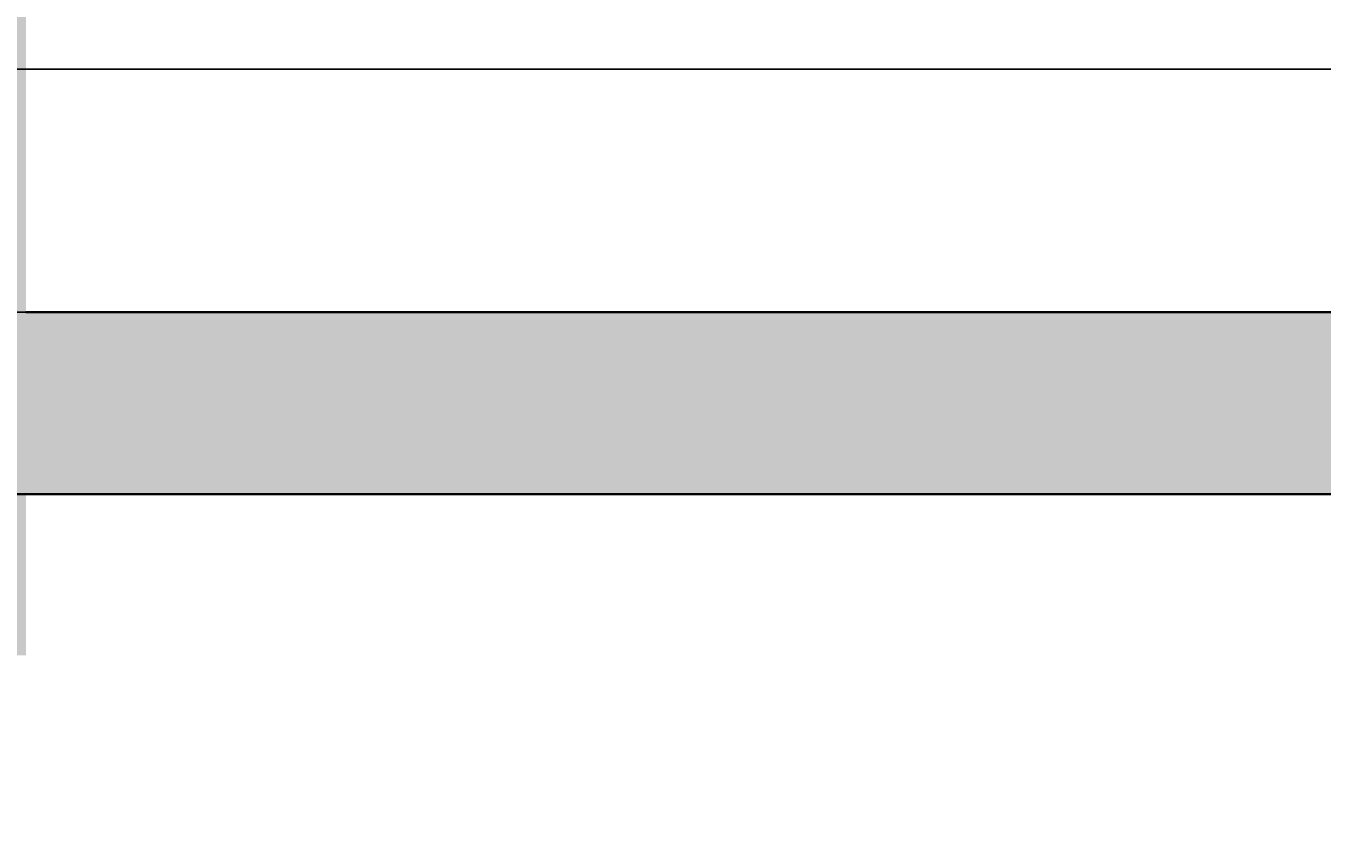
# Model space of a CAD drawing. Units: inches. Extents: x 1998 to 2588, y 1139 to 1977.
# Tile 10 of 134: x 2115 to 2147, y 1576 to 1596. Entities that reach past the tile are written whole.
import ezdxf

# ---------------------------------------------------------------- set-up
doc = ezdxf.new("R2010")
doc.units = ezdxf.units.IN
for name, color, linetype, lineweight in [('A-ANNO-DIMS', 2, 'Continuous', 18), ('A-WALL-PATT', 252, 'Continuous', 13), ('WALL', 200, 'Continuous', 35)]:
    doc.layers.add(name, color=color, linetype=linetype, lineweight=lineweight)
doc.styles.get("Standard").update_dxf_attribs({"font": 'arial.ttf'})
doc.dimstyles.get("Standard").update_dxf_attribs({"dimtxt": 0.18, "dimasz": 0.18, "dimexe": 0.18, "dimexo": 0.0625, "dimgap": 0.09, "dimtad": 0, "dimtih": 1, "dimtoh": 1, "dimdec": 4, "dimzin": 0, "dimdsep": 46, "dimtxsty": 'Standard', "dimcen": 0.09, "dimadec": 0, "dimazin": 0, "dimtfac": 1, "dimtdec": 4, "dimtofl": 0, "dimtmove": 0, "dimatfit": 3, "dimfxl": 1, "dimtolj": 1, "dimtzin": 0, "dimarcsym": 0})

# ---------------------------------------------------------------- blocks, each defined once
blk = doc.blocks.new('*D30')
at = {"layer": 'A-ANNO-DIMS', "color": 0, "lineweight": -2, "transparency": 16777216}
for p, q in [((2407.91, 1636.732), (1997.843, 1636.732)), ((1998.023, 1636.552), (1998.023, 1615.913)), ((1998.023, 1594.912), (1998.023, 1615.552)), ((2407.91, 1594.732), (1997.843, 1594.732))]:
    blk.add_line(p, q, dxfattribs=at)
at = {"layer": 'A-ANNO-DIMS', "color": 0, "transparency": 16777216}
for points in [[(1997.993, 1636.552), (1998.053, 1636.552), (1998.023, 1636.732)], [(1997.993, 1594.912), (1998.053, 1594.912), (1998.023, 1594.732)]]:
    blk.add_solid(points, dxfattribs=at)
at = {"layer": 'Defpoints', "color": 0, "transparency": 16777216}
for p in [(1998.023, 1636.732), (2407.973, 1636.732), (2407.973, 1594.732)]:
    blk.add_point(p, dxfattribs=at)
at = {"layer": 'A-ANNO-DIMS', "color": 0, "transparency": 16777216, "insert": (1998.023, 1615.732), "char_height": 0.18, "attachment_point": 5}
blk.add_mtext('\\A1;42', dxfattribs=at)
blk = doc.blocks.new('*D34')
at = {"layer": 'A-ANNO-DIMS', "color": 0, "lineweight": -2, "transparency": 16777216}
for p, q in [((2407.91, 1594.732), (1997.843, 1594.732)), ((1998.023, 1594.552), (1998.023, 1558.913)), ((1998.023, 1522.912), (1998.023, 1558.552)), ((2407.91, 1522.732), (1997.843, 1522.732))]:
    blk.add_line(p, q, dxfattribs=at)
at = {"layer": 'A-ANNO-DIMS', "color": 0, "transparency": 16777216}
for points in [[(1997.993, 1594.552), (1998.053, 1594.552), (1998.023, 1594.732)], [(1997.993, 1522.912), (1998.053, 1522.912), (1998.023, 1522.732)]]:
    blk.add_solid(points, dxfattribs=at)
at = {"layer": 'Defpoints', "color": 0, "transparency": 16777216}
for p in [(1998.023, 1594.732), (2407.973, 1594.732), (2407.973, 1522.732)]:
    blk.add_point(p, dxfattribs=at)
at = {"layer": 'A-ANNO-DIMS', "color": 0, "transparency": 16777216, "insert": (1998.023, 1558.732), "char_height": 0.18, "attachment_point": 5}
blk.add_mtext('\\A1;72', dxfattribs=at)
blk = doc.blocks.new('*D35')
at = {"layer": 'A-ANNO-DIMS', "color": 0, "lineweight": -2, "transparency": 16777216}
for p, q in [((2148.392, 1612.732), (1997.843, 1612.732)), ((1998.023, 1612.552), (1998.023, 1600.913)), ((1998.023, 1588.912), (1998.023, 1600.552)), ((2148.392, 1588.732), (1997.843, 1588.732))]:
    blk.add_line(p, q, dxfattribs=at)
at = {"layer": 'A-ANNO-DIMS', "color": 0, "transparency": 16777216}
for points in [[(1997.993, 1612.552), (1998.053, 1612.552), (1998.023, 1612.732)], [(1997.993, 1588.912), (1998.053, 1588.912), (1998.023, 1588.732)]]:
    blk.add_solid(points, dxfattribs=at)
at = {"layer": 'Defpoints', "color": 0, "transparency": 16777216}
for p in [(1998.023, 1612.732), (2148.455, 1612.732), (2148.455, 1588.732)]:
    blk.add_point(p, dxfattribs=at)
at = {"layer": 'A-ANNO-DIMS', "color": 0, "transparency": 16777216, "insert": (1998.023, 1600.732), "char_height": 0.18, "attachment_point": 5}
blk.add_mtext('\\A1;24', dxfattribs=at)

msp = doc.modelspace()

# ---------------------------------------------------------------- hatches: boundary and pattern name
at = {"layer": 'A-WALL-PATT'}
h = msp.add_hatch(color=256, dxfattribs=at)
h.dxf.hatch_style = 1
h.paths.add_polyline_path([(2222.9729, 1888.7324), (2099.4125, 1888.7324), (2099.4125, 1879.7324), (2222.9729, 1879.7324)])
h.paths.add_polyline_path([(2096.9729, 1868.3278), (2087.9729, 1868.3278), (2087.9729, 1775.637), (2096.9729, 1775.637)])
h.paths.add_polyline_path([(2227.4729, 1868.3278), (2222.9729, 1868.3278), (2222.9729, 1774.3318), (2227.4729, 1774.3318)])
h.paths.add_polyline_path([(2188.3019, 1759.7324), (2138.6074, 1759.7324), (2099.4125, 1759.7324), (2099.4125, 1755.2324), (2176.9729, 1755.2324), (2188.3019, 1755.2324)])
h.paths.add_polyline_path([(2087.9729, 1759.7324), (2059.4729, 1759.7324), (2059.4729, 1702.7324), (2087.9729, 1702.7324), (2087.9729, 1707.2324), (2063.9729, 1707.2324), (2063.9729, 1755.2324), (2087.9729, 1755.2324)])
h.paths.add_polyline_path([(2096.9729, 1755.2324), (2087.9729, 1755.2324), (2087.9729, 1707.2324), (2096.9729, 1707.2324)])
h.paths.add_polyline_path([(2187.0461, 1707.2324), (2105.9729, 1707.2324), (2096.9729, 1707.2324), (2087.9729, 1707.2324), (2087.9729, 1702.7324), (2105.9729, 1702.7324), (2114.9729, 1702.7324), (2187.0461, 1702.7324)])
h.paths.add_polyline_path([(2181.4729, 1719.2028), (2176.9729, 1719.2028), (2176.9729, 1707.2324), (2181.4729, 1707.2324)])
h.paths.add_polyline_path([(2216.0332, 1588.7324), (2114.9729, 1588.7324), (2105.9729, 1588.7324), (2105.9729, 1584.2324), (2216.0332, 1584.2324)])
h.paths.add_polyline_path([(2077.691, 1588.7324), (2061.4729, 1588.7324), (2061.4729, 1584.2324), (2077.691, 1584.2324)])
h.paths.add_polyline_path([(2105.9729, 1588.7324), (2098.0956, 1588.7324), (2098.0956, 1584.2324), (2105.9729, 1584.2324)])
h.paths.add_polyline_path([(2114.9729, 1596.2642), (2110.1012, 1596.2642), (2105.9729, 1596.2642), (2105.9729, 1588.7324), (2114.9729, 1588.7324)])
h.paths.add_polyline_path([(2114.9729, 1584.2324), (2105.9729, 1584.2324), (2105.9729, 1580.249), (2110.1012, 1580.249), (2114.9729, 1580.249)])
h.paths.add_polyline_path([(2114.9729, 1547.7716), (2110.1012, 1547.7716, -0.0318759), (2105.9729, 1548.035), (2105.9729, 1470.2324), (2108.3775, 1470.2324), (2108.3775, 1465.7324), (2186.2943, 1465.7324), (2186.2943, 1470.2324), (2114.9729, 1470.2324)])
h.paths.add_polyline_path([(2227.4729, 1584.2324), (2222.9729, 1584.2324), (2222.9729, 1486.137), (2227.4729, 1486.137)])
h.paths.add_polyline_path([(2295.4138, 1593.2324), (2227.4729, 1593.2324), (2227.4729, 1588.7324), (2295.4138, 1588.7324), (2295.4138, 1591.8729)])
h.paths.add_polyline_path([(2345.9729, 1627.1165), (2341.4729, 1627.1165), (2341.4729, 1593.2324), (2337.2869, 1593.2324), (2337.2869, 1591.8729), (2337.2869, 1588.7324), (2345.9729, 1588.7324)])
h.paths.add_polyline_path([(2291.9729, 1588.7324), (2287.4729, 1588.7324), (2287.4729, 1522.7324), (2291.9729, 1522.7324)])
h.paths.add_polyline_path([(2291.9729, 1522.7324), (2287.4729, 1522.7324), (2227.4729, 1522.7324), (2227.4729, 1518.2324), (2291.9729, 1518.2324)])
h.paths.add_polyline_path([(2295.7347, 1519.5919), (2295.7347, 1522.7324), (2291.9729, 1522.7324), (2291.9729, 1518.2324), (2295.7347, 1518.2324)])
h.paths.add_polyline_path([(2345.9729, 1522.7324), (2337.6078, 1522.7324), (2337.6078, 1519.5919), (2337.6078, 1518.2324), (2341.4729, 1518.2324), (2341.4729, 1488.5616), (2345.9729, 1488.5616)])
h.paths.add_polyline_path([(2345.9729, 1468.1569), (2341.4729, 1468.1569), (2341.4729, 1374.2324), (2227.4729, 1374.2324), (2227.4729, 1369.7324), (2345.9729, 1369.7324)])
h.paths.add_polyline_path([(2345.9729, 1369.7324), (2341.4729, 1369.7324), (2341.4729, 1362.2324), (2345.9729, 1362.2324)])
h.paths.add_polyline_path([(2345.9729, 1317.7324), (2345.9729, 1322.2324), (2341.4729, 1322.2324), (2341.4729, 1285.137), (2345.9729, 1285.137)], flags=17)
h.paths.add_polyline_path([(2356.2096, 1322.2324), (2345.9729, 1322.2324), (2345.9729, 1317.7324), (2356.2096, 1317.7324), (2356.2096, 1319.3088)], flags=17)
h.paths.add_polyline_path([(2393.9729, 1322.2324), (2375.6999, 1322.2324), (2375.6999, 1319.3088, -0.0202458), (2375.636, 1317.7324), (2393.9729, 1317.7324)], flags=17)
h.paths.add_polyline_path([(2398.4729, 1322.2324), (2393.9729, 1322.2324), (2393.9729, 1317.7324), (2393.9729, 1237.7324), (2345.9729, 1237.7324), (2345.9729, 1264.7324), (2341.4729, 1264.7324), (2341.4729, 1228.7324), (2393.9729, 1228.7324), (2482.7412, 1228.7324), (2482.7412, 1237.7324), (2398.4729, 1237.7324), (2398.4729, 1297.1029)])
h.paths.add_polyline_path([(2398.4729, 1362.2324), (2393.9729, 1362.2324), (2393.9729, 1357.7324), (2398.4729, 1357.7324)])
h.paths.add_polyline_path([(2345.9729, 1329.7549), (2341.4729, 1329.7549), (2341.4729, 1322.2324), (2345.9729, 1322.2324)])

# ---------------------------------------------------------------- linework, layer by layer
at = {"layer": 'WALL'}
for p, q in [((2216.0332, 1588.7324), (2114.9729, 1588.7324)), ((2227.4729, 1584.2324), (2105.9729, 1584.2324))]:
    msp.add_line(p, q, dxfattribs=at)

# ---------------------------------------------------------------- dimensions: what is measured, and where the dimension line sits
at = {"layer": 'A-ANNO-DIMS'}
for base, p1, p2, picture, middle in [((1998.0229, 1636.7324), (2407.9729, 1594.7324), (2407.9729, 1636.7324), '*D30', (1998.0229, 1615.7324)), ((1998.0229, 1612.7324), (2148.4548, 1588.7324), (2148.4548, 1612.7324), '*D35', (1998.0229, 1600.7324)), ((1998.0229, 1594.7324), (2407.9729, 1522.7324), (2407.9729, 1594.7324), '*D34', (1998.0229, 1558.7324))]:
    dim = msp.add_linear_dim(base=base, p1=p1, p2=p2, angle=90, dimstyle='Standard', override={"dimdec": 0, "dimlfac": 1, "dimrnd": 0, "dimzin": 0, "dimdsep": 46, "dimlunit": 2}, dxfattribs=at)
    dim.commit()
    dim.dimension.update_dxf_attribs({"geometry": picture, "text_midpoint": middle})

doc.saveas('drawing.dxf')
